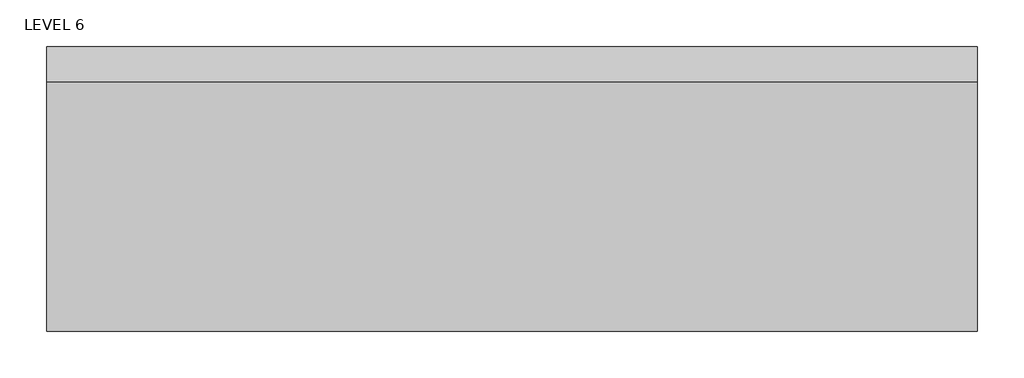
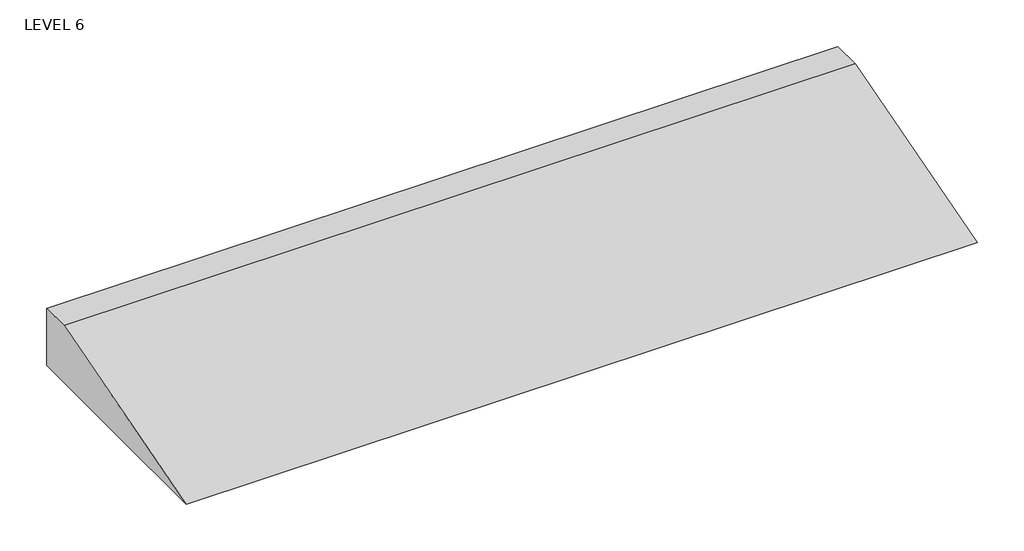
# One storey: 1 proxy.
"""IFC4 building model written with IfcOpenShell, lengths in millimetres."""

from ifc_helpers import new_model, si_unit, origin, place, context, project, spatial, transform, mapped, element, save
from components import generic_models_11_generic_models_11_be4b57fd

model = new_model("IFC4")

# Units and contexts
model_context = context("Model", 3, world=origin())
ifc_project = project(units=[si_unit("LENGTHUNIT", "METRE", prefix="MILLI")], contexts=[model_context])

# Site, building, storey
site = spatial("IfcSite", under=ifc_project)
building = spatial("IfcBuilding", under=site)
storey = spatial("IfcBuildingStorey", under=building, Name="LEVEL 6", Elevation=-609.6)

# Proxy
placement = place(None, origin())
generic_models_11_generic_models_11_shape = generic_models_11_generic_models_11_be4b57fd(model_context)
element("IfcBuildingElementProxy", 1, Name="Generic Models 11 : Generic Models 11", ObjectType="Generic Models 11 : Generic Models 11", at=placement, inside=storey, context=model_context, shape_type="MappedRepresentation", body=[
    mapped(generic_models_11_generic_models_11_shape, transform((0.0, 0.0, 0.0), x_axis=(1.0, 0.0, 0.0), y_axis=(0.0, 1.0, 0.0), z_axis=(0.0, 0.0, 1.0))),
])

save(model, "model.ifc")

# Revit data of these elements
# Element 1 (IfcBuildingElementProxy, "Generic Models 11 : Generic Models 11")
#   Phase Created = New Construction
